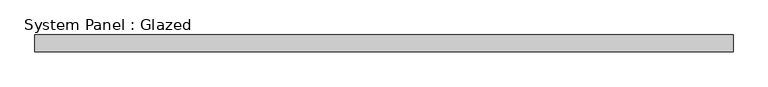
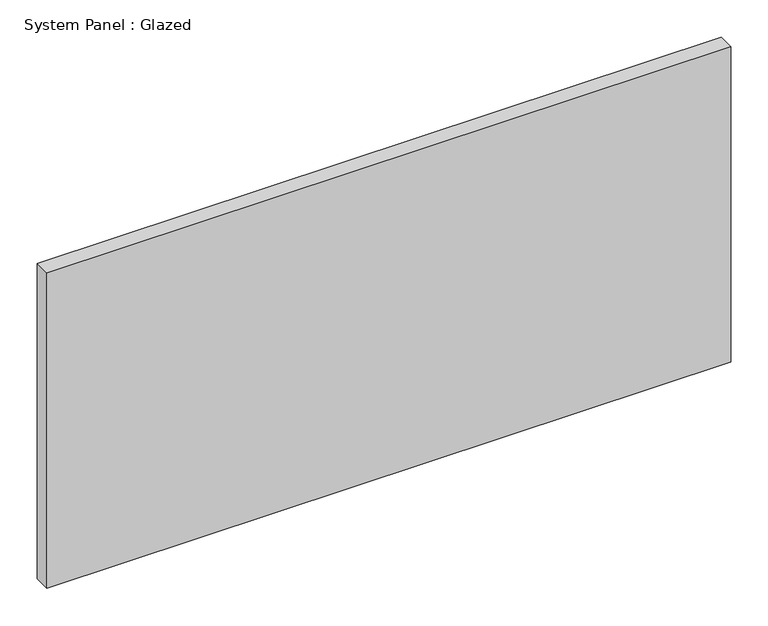
"""IFC4 building model written with IfcOpenShell, lengths in millimetres: plate geometry, System Panel : Glazed."""

from ifc_helpers import new_model, si_unit, origin, origin_with_axes, place, context, project, spatial, polyline, outline, extrude, source, transform, mapped, element, save


def system_panel_glazed_40ca61d7(model_context):
    return source(origin(), model_context, "Body", "SweptSolid", [
        extrude(outline(polyline([(527.05, 19.05), (-527.05, 19.05), (-527.05, 44.45), (527.05, 44.45), (527.05, 19.05)])), origin_with_axes(), (0.0, 0.0, 1.0), 514.35),
    ])


if __name__ == "__main__":
    model = new_model("IFC4")
    model_context = context("Model", 3, world=origin())
    ifc_project = project(units=[si_unit("LENGTHUNIT", "METRE", prefix="MILLI")], contexts=[model_context])
    site = spatial("IfcSite", under=ifc_project)
    building = spatial("IfcBuilding", under=site)
    placement = place(None, origin())
    system_panel_glazed_shape = system_panel_glazed_40ca61d7(model_context)
    element("IfcPlate", 1, ObjectType="System Panel : Glazed", at=placement, inside=building, context=model_context, shape_type="MappedRepresentation", body=[
        mapped(system_panel_glazed_shape, transform((0.0, 0.0, 0.0), x_axis=(1.0, 0.0, 0.0), y_axis=(0.0, 1.0, 0.0), z_axis=(0.0, 0.0, 1.0))),
    ])
    save(model, "model.ifc")

# Revit data of these elements
# Type "System Panel : Glazed"
#   Construction Type Id = "GSP4R"
#   Analytic Construction = "1/8 in Pilkington single glazing"
#   Visual Light Transmittance = 0.9
#   Solar Heat Gain Coefficient = 0.86
#   Heat Transfer Coefficient (U) = 1.18115 BTU/(h·ft²·°F)
# Element 1 (IfcPlate, "System Panel : Glazed")
#   Materials on its faces: "Glass"
# Materials
#   "Glass": class "Glass", colour RGB 0 128 192, transparency 0.75, Description = "Soda Lime Glass", Cost = 0
